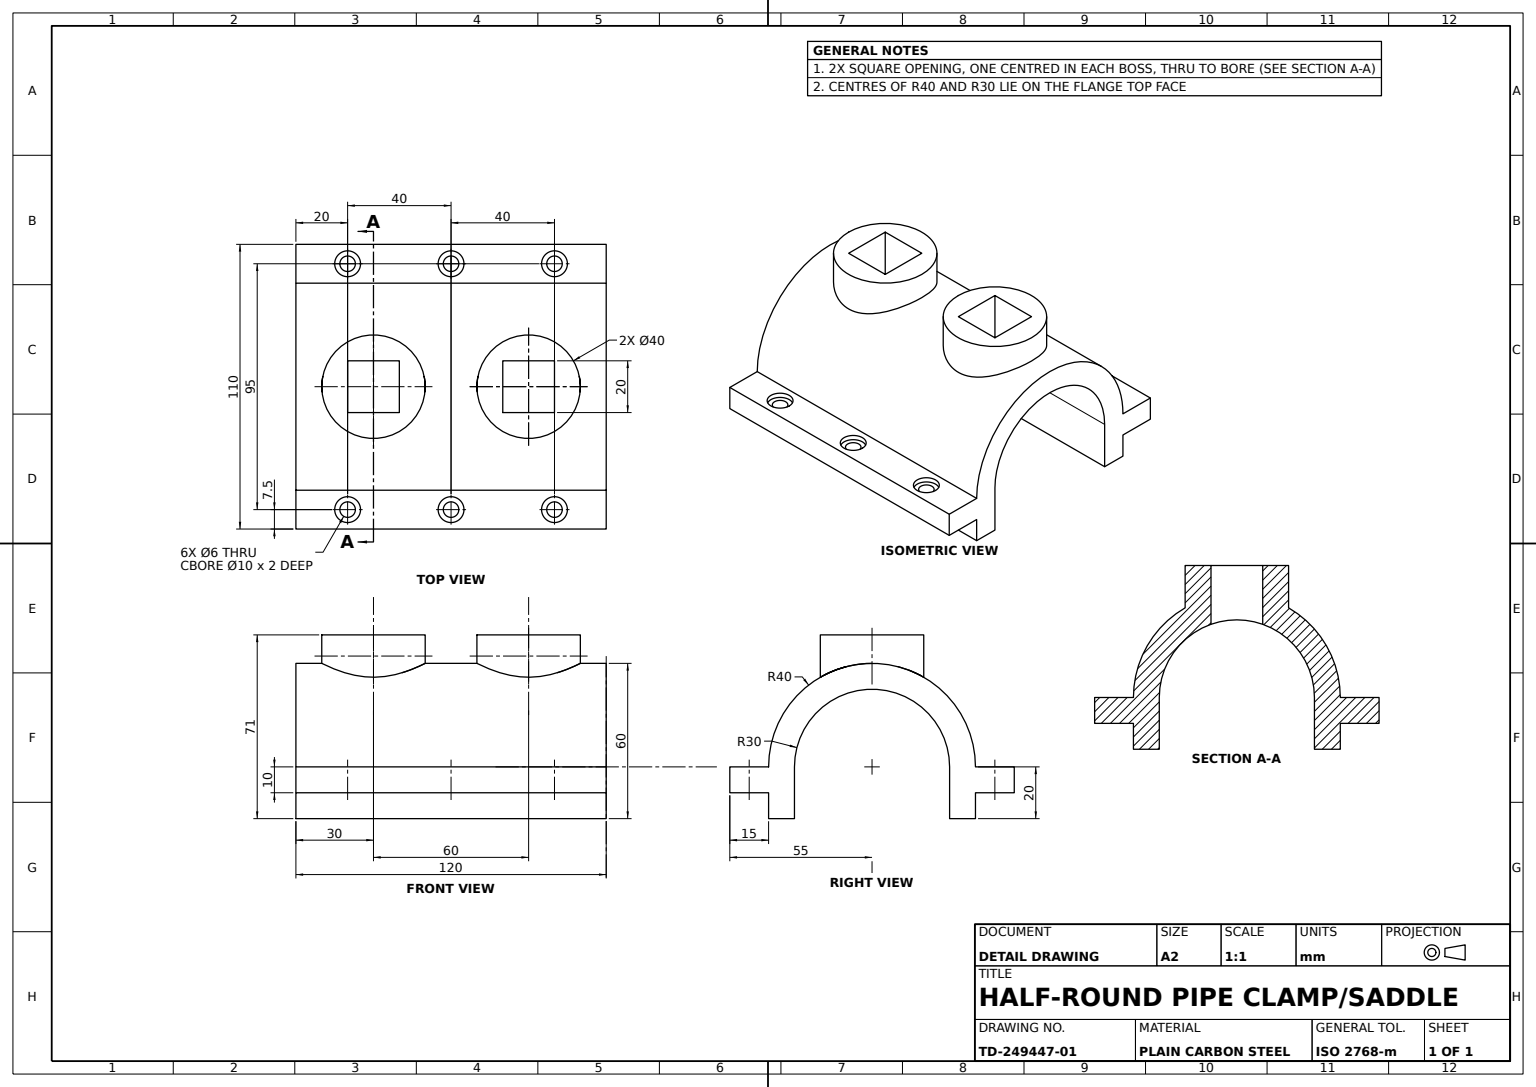
from build123d import *

# Parameters (mm, degrees)
HALF_PIPE_CAP_BODY_DEPTH     = 120
MOUNTING_HOLES_SKETCH_R      = 3
MOUNTING_HOLES_6X_6_DEPTH    = 120
COUNTERBORE_SKETCH_R         = 5
COUNTERBORE_SKETCH_R_2       = 3
COUNTERBORES_6X_10X2_DEPTH   = 2
BOSS_SKETCH_R                = 20
BOSS_SKETCH_W                = 20
BOSS_SKETCH_H                = 20
TOP_BOSSES_2X_40_DEPTH       = 20
SQUARE_SOCKET_SKETCH_W       = 20
SQUARE_SOCKET_SKETCH_H       = 20
SQUARE_SOCKETS_2X20X20_DEPTH = 20


with BuildPart() as part:
    # Cap Profile Sketch → Half Pipe Cap Body (new body)
    with BuildSketch(Plane.XY):
        with BuildLine():
            Line((-55, 0), (-40, 0))
            ThreePointArc((-40, 0), (0, 40), (40, 0))
            Line((40, 0), (55, 0))
            Line((55, 0), (55, -10))
            Line((55, -10), (40, -10))
            Line((40, -10), (40, -20))
            Line((40, -20), (30, -20))
            Line((30, -20), (30, 0))
            ThreePointArc((30, 0), (0, 30), (-30, 0))
            Line((-30, 0), (-30, -20))
            Line((-30, -20), (-40, -20))
            Line((-40, -20), (-40, -10))
            Line((-40, -10), (-55, -10))
            Line((-55, -10), (-55, 0))
        make_face()
    extrude(amount=HALF_PIPE_CAP_BODY_DEPTH)

    # Mounting Holes Sketch → Mounting Holes 6xØ6 (cut)
    with BuildSketch(Plane(origin=(0, 0, 0), x_dir=(1, 0, 0), z_dir=(0, 1, 0))):
        with Locations(Location((-47.5, -20, 0), (0, 0, 270))):
            Circle(MOUNTING_HOLES_SKETCH_R)
        with Locations(Location((-47.5, -100, 0), (0, 0, 270))):
            Circle(MOUNTING_HOLES_SKETCH_R)
        with Locations(Location((-47.5, -60, 0), (0, 0, 270))):
            Circle(MOUNTING_HOLES_SKETCH_R)
        with Locations(Location((47.5, -20, 0), (0, 0, 270))):
            Circle(MOUNTING_HOLES_SKETCH_R)
        with Locations(Location((47.5, -60, 0), (0, 0, 270))):
            Circle(MOUNTING_HOLES_SKETCH_R)
        with Locations(Location((47.5, -100, 0), (0, 0, 270))):
            Circle(MOUNTING_HOLES_SKETCH_R)
    extrude(amount=-MOUNTING_HOLES_6X_6_DEPTH, mode=Mode.SUBTRACT)

    # Counterbore Sketch → Counterbores 6xØ10x2 (cut)
    # profile 1 of 6: a face of its own
    with BuildSketch(Plane(origin=(0, 0, 0), x_dir=(1, 0, 0), z_dir=(0, 1, 0))):
        with Locations(Location((-47.5, -60, 0), (0, 0, 270))):
            Circle(COUNTERBORE_SKETCH_R)
        with Locations(Location((-47.5, -60, 0), (0, 0, 270))):
            Circle(COUNTERBORE_SKETCH_R_2, mode=Mode.SUBTRACT)
    # profile 2 of 6: a face of its own
    with BuildSketch(Plane(origin=(0, 0, 0), x_dir=(1, 0, 0), z_dir=(0, 1, 0))):
        with Locations(Location((-47.5, -100, 0), (0, 0, 270))):
            Circle(COUNTERBORE_SKETCH_R)
        with Locations(Location((-47.5, -100, 0), (0, 0, 270))):
            Circle(COUNTERBORE_SKETCH_R_2, mode=Mode.SUBTRACT)
    # profile 3 of 6: a face of its own
    with BuildSketch(Plane(origin=(0, 0, 0), x_dir=(1, 0, 0), z_dir=(0, 1, 0))):
        with Locations(Location((-47.5, -20, 0), (0, 0, 270))):
            Circle(COUNTERBORE_SKETCH_R)
        with Locations(Location((-47.5, -20, 0), (0, 0, 270))):
            Circle(COUNTERBORE_SKETCH_R_2, mode=Mode.SUBTRACT)
    # profile 4 of 6: a face of its own
    with BuildSketch(Plane(origin=(0, 0, 0), x_dir=(1, 0, 0), z_dir=(0, 1, 0))):
        with Locations(Location((47.5, -20, 0), (0, 0, 270))):
            Circle(COUNTERBORE_SKETCH_R)
        with Locations(Location((47.5, -20, 0), (0, 0, 270))):
            Circle(COUNTERBORE_SKETCH_R_2, mode=Mode.SUBTRACT)
    # profile 5 of 6: a face of its own
    with BuildSketch(Plane(origin=(0, 0, 0), x_dir=(1, 0, 0), z_dir=(0, 1, 0))):
        with Locations(Location((47.5, -60, 0), (0, 0, 270))):
            Circle(COUNTERBORE_SKETCH_R)
        with Locations(Location((47.5, -60, 0), (0, 0, 270))):
            Circle(COUNTERBORE_SKETCH_R_2, mode=Mode.SUBTRACT)
    # profile 6 of 6: a face of its own
    with BuildSketch(Plane(origin=(0, 0, 0), x_dir=(1, 0, 0), z_dir=(0, 1, 0))):
        with Locations(Location((47.5, -100, 0), (0, 0, 270))):
            Circle(COUNTERBORE_SKETCH_R)
        with Locations(Location((47.5, -100, 0), (0, 0, 270))):
            Circle(COUNTERBORE_SKETCH_R_2, mode=Mode.SUBTRACT)
    extrude(amount=-COUNTERBORES_6X_10X2_DEPTH, mode=Mode.SUBTRACT)

    # Boss Sketch → Top Bosses 2xØ40 (add)
    # profile 1 of 2: a face of its own
    with BuildSketch(Plane(origin=(0, 31, 0), x_dir=(1, 0, 0), z_dir=(0, 1, 0))):
        with Locations(Location((0, -30, 0), (0, 0, 90))):
            Circle(BOSS_SKETCH_R)
        with Locations((0, -30)):
            Rectangle(BOSS_SKETCH_W, BOSS_SKETCH_H, mode=Mode.SUBTRACT)
    # profile 2 of 2: a face of its own
    with BuildSketch(Plane(origin=(0, 31, 0), x_dir=(1, 0, 0), z_dir=(0, 1, 0))):
        with Locations(Location((0, -90, 0), (0, 0, 90))):
            Circle(BOSS_SKETCH_R)
        with Locations((0, -90)):
            Rectangle(BOSS_SKETCH_W, BOSS_SKETCH_H, mode=Mode.SUBTRACT)
    extrude(amount=TOP_BOSSES_2X_40_DEPTH)

    # Square Socket Sketch → Square Sockets 2x20x20 (cut, symmetric)
    with BuildSketch(Plane(origin=(0, 31, 0), x_dir=(1, 0, 0), z_dir=(0, 1, 0))):
        with Locations((0, -30)):
            Rectangle(SQUARE_SOCKET_SKETCH_W, SQUARE_SOCKET_SKETCH_H)
        with Locations((0, -90)):
            Rectangle(SQUARE_SOCKET_SKETCH_W, SQUARE_SOCKET_SKETCH_H)
    extrude(amount=SQUARE_SOCKETS_2X20X20_DEPTH, both=True, mode=Mode.SUBTRACT)


solid = part.part
